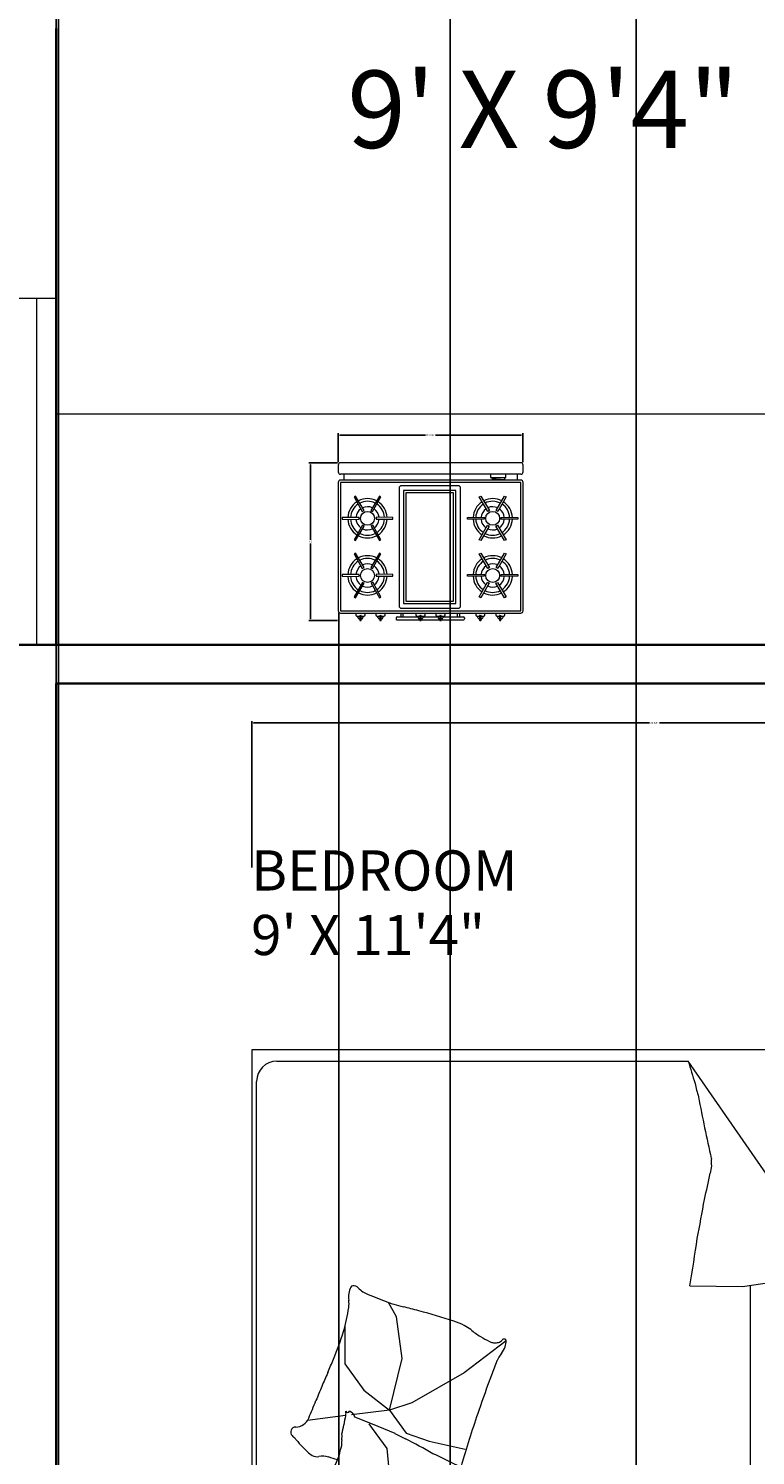
# Model space of a CAD drawing. Units: feet. Extents: x 1993 to 2298, y 2938 to 3641.
# Tile 6 of 11: x 2147 to 2222, y 3144 to 3293. Entities that reach past the tile are written whole.
import ezdxf

# ---------------------------------------------------------------- set-up
doc = ezdxf.new("R2010")
doc.units = ezdxf.units.FT
for name, color, linetype, lineweight in [('A-ANNO-DIMS', 2, 'Continuous', 18), ('A-AREA-IDEN', 7, 'Continuous', 18), ('A-EQPM', 8, 'Continuous', 18), ('A-FLOR-CASE', 8, 'Continuous', 18), ('A-GLAZ', 4, 'Continuous', 13), ('furniture', 8, 'Continuous', 18), ('WAL', 7, 'Continuous', 35)]:
    doc.layers.add(name, color=color, linetype=linetype, lineweight=lineweight)
doc.styles.add('DIM_FONT', font='SIMPLEX.shx', dxfattribs={"width": 0.8})
doc.styles.get("Standard").update_dxf_attribs({"font": 'arial.ttf'})
doc.dimstyles.get("Standard").update_dxf_attribs({"dimtxt": 0.18, "dimasz": 0.18, "dimexe": 0.18, "dimexo": 0.0625, "dimgap": 0.09, "dimtad": 0, "dimtih": 1, "dimtoh": 1, "dimdec": 4, "dimzin": 0, "dimdsep": 46, "dimtxsty": 'Standard', "dimcen": 0.09, "dimadec": 0, "dimazin": 0, "dimtfac": 1, "dimtdec": 4, "dimtofl": 0, "dimtmove": 0, "dimatfit": 3, "dimfxl": 1, "dimtolj": 1, "dimtzin": 0, "dimarcsym": 0})

# ---------------------------------------------------------------- blocks, each defined once
blk = doc.blocks.new('A$C79766A75')
for p, q in [((0.45, 1.9999), (0, 1.9999)), ((0, 1.9999), (0, 1.5499)), ((0.45, 1.5499), (0.45, 1.9999)), ((1.9506, 2), (0.4506, 2)), ((0.4506, 2), (0.4506, 0)), ((1.9506, 0), (1.9506, 2)), ((2.402, 1.9999), (1.952, 1.9999)), ((1.952, 1.9999), (1.952, 1.5499)), ((2.402, 1.5499), (2.402, 1.9999)), ((0.42, 1.9699), (0.03, 1.9699)), ((0.03, 1.9699), (0.03, 1.5799)), ((0.42, 1.5799), (0.42, 1.9699)), ((2.372, 1.9699), (1.982, 1.9699)), ((1.982, 1.9699), (1.982, 1.5799)), ((2.372, 1.5799), (2.372, 1.9699)), ((0.2304, 1.9125), (0.2304, 1.6061)), ((1.9506, 1.9476), (0.4506, 1.9476)), ((2.1824, 1.9125), (2.1824, 1.6061)), ((0.0743, 1.7595), (0.3834, 1.7595)), ((2.0263, 1.7595), (2.3354, 1.7595)), ((1.1461, 1.5617), (1.1254, 1.6443)), ((1.8553, 1.5617), (1.8346, 1.6443)), ((0.4234, 1.6034), (0.4228, 1.6034)), ((0.03, 1.5799), (0.42, 1.5799)), ((1.1536, 1.5317), (1.1461, 1.5617)), ((1.8628, 1.5317), (1.8553, 1.5617)), ((1.982, 1.5799), (2.372, 1.5799)), ((0, 1.5499), (0.45, 1.5499)), ((1.952, 1.5499), (2.402, 1.5499)), ((1.0972, 1.5115), (0.4791, 1.0841)), ((1.0972, 1.5115), (1.9048, 1.5115)), ((1.9248, 1.4915), (1.9248, 0.0322)), ((1.0383, 1.2184), (1.0246, 1.3138)), ((1.9048, 1.2389), (1.0354, 1.2389)), ((1.0365, 1.0883), (1.0383, 1.2184)), ((0.4791, 0.0622), (0.4791, 1.0841)), ((1.1731, 0.6316), (1.2523, 0.5276)), ((1.5696, 0.6317), (1.5559, 0.5286)), ((1.2523, 0.5276), (1.3274, 0.3973)), ((1.4223, 0.4407), (1.442, 0.5296)), ((1.5559, 0.5286), (1.5817, 0.4065)), ((1.6952, 0.4478), (1.7898, 0.4856)), ((1.7898, 0.4856), (1.8139, 0.4822)), ((1.4025, 0.3834), (1.4223, 0.4407)), ((1.6264, 0.355), (1.6952, 0.4478)), ((1.3274, 0.3973), (1.3452, 0.342)), ((1.5817, 0.4065), (1.6264, 0.355)), ((1.1139, 0.3597), (1.0779, 0.3397)), ((1.2167, 0.3736), (1.1139, 0.3597)), ((1.3452, 0.342), (1.2167, 0.3736)), ((1.3452, 0.342), (1.4025, 0.3834)), ((1.4034, 0.3558), (1.3803, 0.2995)), ((1.6264, 0.355), (1.4406, 0.3361)), ((1.5954, 0.2725), (1.6264, 0.355)), ((1.6264, 0.355), (1.6935, 0.3825)), ((1.6935, 0.3825), (1.7623, 0.379)), ((1.7623, 0.379), (1.8603, 0.3619)), ((1.8603, 0.3619), (1.8636, 0.3554)), ((1.2957, 0.2787), (1.3452, 0.342)), ((1.3452, 0.342), (1.3569, 0.2478)), ((1.4406, 0.3361), (1.3907, 0.3)), ((1.3803, 0.2995), (1.3626, 0.256)), ((1.3907, 0.3), (1.3787, 0.2914)), ((1.2305, 0.2313), (1.2957, 0.2787)), ((1.6161, 0.19), (1.5954, 0.2725)), ((1.1376, 0.2313), (1.2305, 0.2313)), ((1.3588, 0.2331), (1.3706, 0.1385)), ((1.6697, 0.1274), (1.6161, 0.19)), ((1.9048, 0.0122), (0.5291, 0.0122)), ((0.4506, 0), (1.9506, 0))]:
    blk.add_line(p, q)
for centre in [(0.2304, 1.7595), (2.1824, 1.7595)]:
    blk.add_circle(centre, 0.126)
for centre, radius, start, end in [((0.5232, 1.9139), 0.00342, 291.7883, 340.436), ((0.5246, 1.9378), 0.0251, 274.3025, 291.7883), ((0.5486, 1.9393), 0.0289, 239.3487, 274.3025), ((1.1179, 2.0719), 0.1611, 270, 278.4372), ((1.1592, 2.0011), 0.0904, 258.7276, 270), ((1.2325, 1.9139), 0.00342, 291.7883, 340.436), ((1.2338, 1.9378), 0.0251, 274.3025, 291.7883), ((1.2578, 1.9393), 0.0289, 239.3487, 274.3025), ((1.8271, 2.0719), 0.1611, 270, 278.4372), ((1.8684, 2.0011), 0.0904, 258.7276, 270), ((0.525, 1.9085), 0.00232, 340.436, 101.8931), ((0.5311, 1.9093), 0.00428, 201.9904, 281.8931), ((0.4996, 1.8889), 0.0328, 338.579, 8.1335), ((0.2896, 1.8253), 0.246, 8.1335, 12.1095), ((0.5465, 1.8994), 0.0156, 158.579, 201.9904), ((0.5458, 1.8568), 0.0539, 59.3487, 84.7408), ((0.546, 1.0829), 0.8208, 84.7408, 88.0921), ((0.6118, 2.0005), 0.0992, 254.0648, 274.2159), ((0.6775, 1.9817), 0.0992, 233.9136, 254.0648), ((0.6362, 0.406), 1.4943, 88.0921, 90.5757), ((0.7304, 1.9449), 0.0992, 216.1766, 233.9136), ((0.7737, 2.1075), 0.234, 242.7604, 249.1397), ((0.7591, 1.0293), 0.8732, 90.5757, 94.8018), ((0.738, 1.949), 0.0768, 231.6114, 242.7604), ((0.974, 2.1633), 0.3916, 226.1885, 231.6114), ((0.7631, 2.1919), 0.2897, 267.4614, 274.8018), ((0.8143, 2.0532), 0.1524, 259.8101, 267.4614), ((0.7515, 1.3747), 0.5293, 79.8101, 83.9133), ((0.8451, 0.8466), 1.049, 83.9133, 90), ((1.046, 1.2129), 0.6827, 90, 97.5469), ((1.1117, 1.6625), 0.2422, 97.5469, 105.744), ((1.0352, 2.2041), 0.3048, 278.4372, 285.744), ((1.171, 1.8579), 0.0342, 94.4002, 153.4195), ((1.1709, 1.9049), 0.0131, 153.4195, 258.7276), ((1.2342, 1.9085), 0.00232, 340.436, 101.8931), ((1.2404, 1.9093), 0.00428, 201.9904, 281.8931), ((1.2088, 1.8889), 0.0328, 338.579, 8.1335), ((0.9988, 1.8253), 0.246, 8.1335, 12.1095), ((1.2558, 1.8994), 0.0156, 158.579, 201.9904), ((1.2551, 1.8568), 0.0539, 59.3487, 84.7408), ((1.2552, 1.0829), 0.8208, 84.7408, 88.0921), ((1.3211, 2.0005), 0.0992, 254.0648, 274.2159), ((1.3868, 1.9817), 0.0992, 233.9136, 254.0648), ((1.3455, 0.406), 1.4943, 88.0921, 90.5757), ((1.4396, 1.9449), 0.0992, 216.1766, 233.9136), ((1.4829, 2.1075), 0.234, 242.7604, 249.1397), ((1.4683, 1.0293), 0.8732, 90.5757, 94.8018), ((1.4473, 1.949), 0.0768, 231.6114, 242.7604), ((1.6833, 2.1633), 0.3916, 226.1885, 231.6114), ((1.4724, 2.1919), 0.2897, 267.4614, 274.8018), ((1.5236, 2.0532), 0.1524, 259.8101, 267.4614), ((1.4607, 1.3747), 0.5293, 79.8101, 83.9133), ((1.5543, 0.8466), 1.049, 83.9133, 90), ((1.7552, 1.2129), 0.6827, 90, 97.5469), ((1.821, 1.6625), 0.2422, 97.5469, 105.744), ((1.7444, 2.2041), 0.3048, 278.4372, 285.744), ((1.8802, 1.8579), 0.0342, 94.4002, 153.4195), ((1.8802, 1.9049), 0.0131, 153.4195, 258.7276), ((0.7297, 1.8867), 0.1983, 187.6809, 192.1095), ((1.4472, 1.8987), 0.9131, 183.3687, 187.6809), ((0.7661, 1.8961), 0.0992, 198.4397, 216.1766), ((0.9057, 1.9982), 0.2252, 219.0349, 226.1885), ((1.6324, 1.8735), 0.4918, 180, 186.2324), ((1.4389, 1.8867), 0.1983, 187.6809, 192.1095), ((2.1565, 1.8987), 0.9131, 183.3687, 187.6809), ((1.4753, 1.8961), 0.0992, 198.4397, 216.1766), ((1.615, 1.9982), 0.2252, 219.0349, 226.1885), ((1.6908, 1.9123), 0.1399, 314.9024, 332.6012), ((1.7511, 1.9723), 0.1399, 297.2036, 314.9024), ((1.7896, 1.8667), 0.0526, 318.5571, 334.6449), ((1.784, 1.9167), 0.0899, 306.2641, 318.5571), ((2.3416, 1.8735), 0.4918, 180, 186.2324), ((0.7932, 1.8591), 0.0493, 208.3168, 219.0349), ((0.9392, 1.9062), 0.2002, 203.0028, 208.3168), ((1.3446, 1.7858), 0.204, 170.3156, 180), ((1.5025, 1.8591), 0.0493, 208.3168, 219.0349), ((1.6484, 1.9062), 0.2002, 203.0028, 208.3168), ((1.6554, 1.8529), 0.1399, 332.6012, 343.485), ((1.7653, 1.8132), 0.0562, 341.2201, 0), ((1.6307, 1.8895), 0.2056, 338.1851, 341.2201), ((1.6887, 1.8881), 0.1511, 334.6449, 338.1851), ((2.0538, 1.7858), 0.204, 170.3156, 180), ((1.2208, 1.7573), 0.6787, 178.3669, 183.3687), ((2.0027, 1.5994), 0.882, 167.8016, 170.3156), ((1.9301, 1.7573), 0.6787, 178.3669, 183.3687), ((1.6404, 1.8023), 0.1399, 343.485, 354.3689), ((1.73, 1.7719), 0.0915, 0, 14.6851), ((2.7119, 1.5994), 0.882, 167.8016, 170.3156), ((0.8192, 1.792), 0.3171, 347.8016, 351.9949), ((1.5284, 1.792), 0.3171, 347.8016, 351.9949), ((1.9066, 1.6447), 1.3652, 176.945, 178.3669), ((0.4711, 1.7556), 0.6588, 351.9949, 357.3351), ((2.6158, 1.6447), 1.3652, 176.945, 178.3669), ((1.1803, 1.7556), 0.6588, 351.9949, 357.3351), ((14.1519, 0.85), 13.6356, 176.49514, 176.94504), ((14.8612, 0.85), 13.6356, 176.49514, 176.94504), ((1.0578, 1.6474), 0.0677, 357.3351, 14.0452), ((1.767, 1.6474), 0.0677, 357.3351, 14.0452), ((0.7658, 2.8912), 1.4323, 294.3265, 296.4985), ((1.226, 2.0834), 0.5066, 290.6743, 294.3265), ((1.4305, 1.6796), 0.058, 274.0828, 290.6743), ((1.4679, 1.8969), 0.2721, 266.4448, 274.0828), ((0.8521, 1.5209), 0.3212, 170.0016, 176.4951), ((0.6583, 0.9067), 0.7387, 64.6889, 66.5156), ((0.7015, 0.888), 0.7387, 66.5156, 68.3423), ((0.7501, 0.8688), 0.7387, 68.3423, 70.572), ((1.5613, 1.5209), 0.3212, 170.0016, 176.4951), ((0.9025, 2.1618), 0.7286, 302.135, 305.8263), ((1.1895, 1.8508), 0.3126, 296.4985, 302.135), ((1.3675, 0.9067), 0.7387, 64.6889, 66.5156), ((1.4107, 0.888), 0.7387, 66.5156, 68.3423), ((1.4594, 0.8688), 0.7387, 68.3423, 70.572), ((0.513, 1.535), 0.0193, 350.0016, 16.6978), ((0.5322, 1.5304), 0.00132, 16.6978, 97.1204), ((0.5579, 1.4467), 0.0875, 97.1204, 106.2212), ((0.5822, 1.4654), 0.0767, 106.2212, 117.2841), ((0.5507, 1.5832), 0.0453, 282.869, 297.2841), ((0.5623, 1.6885), 0.1459, 273.574, 282.869), ((0.589, 2.7103), 1.164, 270.2865, 273.574), ((0.7584, 7.2662), 5.7185, 269.0296, 270.2865), ((0.9401, 4.9065), 3.3622, 267.3904, 269.0296), ((0.9811, 2.7573), 1.2165, 265.3824, 267.3904), ((0.8583, 0.139), 1.4048, 85.3824, 87.2509), ((1.0175, 1.3138), 0.2301, 87.2509, 101.5586), ((0.8043, 0.8497), 0.7387, 70.572, 72.8018), ((1.0449, 1.6886), 0.1459, 263.5659, 281.5586), ((1.1099, 1.6599), 0.1197, 252.6136, 263.5659), ((1.0587, 1.3144), 0.2297, 72.6136, 80.5159), ((1.108, 1.2635), 0.2708, 80.5159, 85.9171), ((1.1535, 1.5308), 0.000917, 85.9171, 194.0449), ((1.2222, 1.535), 0.0193, 350.0016, 16.6978), ((1.2414, 1.5304), 0.00132, 16.6978, 97.1204), ((1.2671, 1.4467), 0.0875, 97.1204, 106.2212), ((1.2914, 1.4654), 0.0767, 106.2212, 117.2841), ((1.2599, 1.5832), 0.0453, 282.869, 297.2841), ((1.2716, 1.6885), 0.1459, 273.574, 282.869), ((1.2982, 2.7103), 1.164, 270.2865, 273.574), ((1.4677, 7.2662), 5.7185, 269.0296, 270.2865), ((1.6493, 4.9065), 3.3622, 267.3904, 269.0296), ((1.6903, 2.7573), 1.2165, 265.3824, 267.3904), ((1.5676, 0.139), 1.4048, 85.3824, 87.2509), ((1.7268, 1.3138), 0.2301, 87.2509, 101.5586), ((1.5136, 0.8497), 0.7387, 70.572, 72.8018), ((1.7541, 1.6886), 0.1459, 263.5659, 281.5586), ((1.8192, 1.6599), 0.1197, 252.6136, 263.5659), ((1.7679, 1.3144), 0.2297, 72.6136, 80.5159), ((1.8172, 1.2635), 0.2708, 80.5159, 85.9171), ((1.8627, 1.5308), 0.000917, 85.9171, 194.0449), ((0.745, 1.6407), 0.3751, 320.3555, 339.8512), ((1.9048, 1.4915), 0.02, 0, 90), ((0.8556, 1.3759), 0.1801, 339.8512, 8.1356), ((1.9048, 1.2589), 0.02, 270, 0), ((-0.1888, 5.1029), 4.0646, 280.7276, 282.9255), ((0.7282, 1.1989), 0.0581, 262.2696, 280.7276), ((0.7833, 1.3309), 0.1942, 256.8096, 262.2696), ((0.2481, -1.3253), 2.5158, 76.8096, 78.3259), ((-0.0248, 2.8487), 1.8351, 285.9352, 287.7364), ((0.3872, 1.7415), 0.6574, 282.9255, 285.9352), ((0.3953, -1.4284), 2.588, 78.3259, 80.505), ((0.413, -2.64), 3.7801, 80.505, 82.308), ((1.1752, 0.6267), 0.0063, 166.7192, 233.4208), ((1.1734, 0.6272), 0.00443, 93.9484, 166.7192), ((1.163, 0.6103), 0.0142, 10.4074, 53.4208), ((1.1755, 0.5964), 0.0352, 69.6548, 93.9484), ((1.1011, 0.5989), 0.0771, 2.7286, 10.4074), ((1.1628, 0.6019), 0.0153, 345.4291, 2.7286), ((1.1669, 0.5731), 0.0601, 51.4146, 69.6548), ((1.2538, 0.682), 0.0792, 231.4146, 247.2931), ((1.5463, 1.3811), 0.8371, 247.2931, 249.8713), ((1.383, 0.7705), 0.2176, 307.2151, 313.5224), ((1.1426, 1.1456), 0.6605, 306.2163, 307.2151), ((1.7751, 0.3162), 0.3825, 126.2163, 127.5287), ((1.5806, 0.5924), 0.0452, 127.5287, 134.1274), ((1.5093, 0.6825), 0.0697, 308.8136, 314.1274), ((1.5706, 0.6318), 0.0127, 176.7545, 308.8136), ((1.5621, 0.59), 0.0359, 356.7545, 62.7098), ((0.9961, 0.6678), 0.194, 320.2995, 329.0944), ((0.8605, 0.749), 0.352, 329.0944, 333.1821), ((1.1396, 0.6079), 0.0393, 333.1821, 345.4291), ((3.0113, 5.3783), 5.0942, 249.8713, 250.9164), ((1.5435, 0.5526), 0.0458, 157.5838, 188.0492), ((1.4828, 0.5833), 0.0226, 324.1064, 8.0492), ((1.4519, 0.6426), 0.0774, 313.5224, 324.1064), ((0.2201, -2.1858), 3.0972, 62.7098, 63.5853), ((2.5711, 2.3551), 2.0162, 242.5001, 243.5853), ((1.2077, 0.4922), 0.081, 140.2995, 153.9265), ((2.374, 3.5362), 3.145, 250.9164, 253.3915), ((2.4089, 0.1204), 1.0054, 154.9471, 157.5838), ((4.5245, 5.9445), 6.1019, 242.15178, 242.50014), ((-0.9881, -4.647), 5.8383, 62.15178, 62.50792), ((3.0311, -0.112), 2.003, 162.1604, 164.7375), ((1.3115, 0.4414), 0.1965, 153.9265, 162.1604), ((2.9813, -0.2643), 1.6868, 152.9116, 154.9471), ((1.5084, 0.6341), 0.1166, 253.3915, 259.2634), ((1.5182, -0.068), 0.6236, 62.5079, 69.2514), ((1.7121, 0.0657), 0.43, 69.2514, 77.3748), ((1.8682, 0.4049), 0.063, 77.3748, 93.3881), ((1.8955, 0.5247), 0.0599, 256.9598, 273.3881), ((1.9257, 0.5082), 0.0509, 238.3083, 256.9598), ((2.8096, -0.3311), 1.5652, 150.064, 152.9116), ((1.8435, 0.4743), 0.0755, 310.5086, 333.6668), ((1.9279, 0.441), 0.0168, 130.5086, 180.9614), ((1.9201, 0.4587), 0.0058, 180.9614, 238.3083), ((2.6887, -0.0186), 1.6481, 164.7375, 166.159), ((-0.5166, 1.5491), 2.6619, 333.6668, 334.8268), ((0.5589, 0.5062), 0.5454, 343.6878, 346.159), ((1.2176, 0.4627), 0.2143, 330.064, 337.7645), ((1.3456, 0.5261), 0.5454, 339.2919, 341.7631), ((1.701, 0.4319), 0.1798, 334.8268, 339.2919), ((-1.4109, 1.284), 2.6619, 338.0627, 339.2227), ((0.9098, 0.4035), 0.1798, 339.2227, 343.6878), ((3.4079, -0.2212), 1.6481, 160.3416, 161.7631), ((0.9882, 0.3177), 0.0755, 314.9045, 338.0627), ((3.6966, -0.4634), 2.003, 157.7645, 160.3416), ((1.0533, 0.2524), 0.0168, 134.9045, 185.3572), ((1.0424, 0.2513), 0.0058, 185.3572, 242.7041), ((1.3694, 0.234), 0.0231, 107.1867, 157.7645), ((1.0631, 0.2914), 0.0509, 242.7041, 261.3557), ((1.0645, 0.3003), 0.0599, 261.3557, 277.784), ((1.0811, 0.1786), 0.063, 81.7707, 97.784), ((1.0286, -0.1846), 0.43, 73.6473, 81.7707), ((0.974, -0.3705), 0.6236, 66.9038, 73.6473), ((1.3465, 0.2383), 0.00467, 287.1867, 70.6201), ((1.3486, 0.2247), 0.0092, 70.6201, 94.2593), ((1.3563, 0.267), 0.034, 262.0178, 274.2593), ((1.4091, 0.4221), 0.1955, 255.1193, 262.0178), ((1.358, 0.0507), 0.1794, 75.1193, 82.3216), ((1.4096, 0.153), 0.0712, 82.3216, 94.5118), ((1.4285, 0.2893), 0.0663, 261.8784, 274.5118), ((1.4755, 0.332), 0.1166, 248.9957, 261.8784), ((2.7121, 3.1012), 3.145, 246.5205, 248.9957), ((2.4175, -0.1202), 1.0054, 160.6552, 161.9797), ((-1.0716, -5.1672), 5.8383, 66.54766, 66.9038), ((3.6805, 5.7866), 6.1019, 246.54766, 246.89602), ((1.505, 0.1766), 0.0458, 161.9797, 192.4451), ((1.856, 0.1288), 0.081, 135.9036, 149.5306), ((1.9797, 0.1108), 0.1965, 149.5306, 157.7645), ((2.0773, 2.0287), 2.0162, 246.896, 247.9812), ((0.1602, -2.7118), 3.0972, 67.1056, 67.9812), ((1.3914, 0.1905), 0.0774, 317.9183, 328.5023), ((1.4382, 0.1619), 0.0226, 328.5023, 12.4451), ((3.6993, 4.7998), 5.0942, 245.4754, 246.5205), ((1.4661, 0.3294), 0.352, 324.6985, 328.7862), ((1.6279, 0.2819), 0.194, 315.9036, 324.6985), ((1.3512, 0.1084), 0.0359, 1.1504, 67.1056), ((1.3997, 0.1094), 0.0127, 181.1504, 313.2095), ((1.4468, 0.0748), 0.0452, 131.9246, 138.5233), ((1.6722, -0.1762), 0.3825, 130.6122, 131.9246), ((0.9933, 0.6156), 0.6605, 310.6122, 311.611), ((1.2874, 0.2845), 0.2176, 311.611, 317.9183), ((2.051, 0.8725), 0.8371, 242.8972, 245.4754), ((1.7576, 0.1689), 0.0792, 227.0187, 242.8972), ((1.7345, 0.1188), 0.0153, 341.0332, 358.3327), ((1.6723, 0.1058), 0.0771, 358.3327, 6.0115), ((1.7162, 0.1388), 0.0393, 328.7862, 341.0332), ((1.3607, 0.1509), 0.0697, 313.2095, 318.5233), ((1.6963, 0.0438), 0.0601, 47.0187, 65.2589), ((1.737, 0.0526), 0.0352, 65.2589, 89.5525), ((1.7401, 0.0928), 0.0142, 6.0115, 49.0249), ((1.756, 0.0832), 0.00443, 89.5525, 162.3233), ((1.7602, 0.0924), 0.0063, 162.3233, 229.0249), ((0.5291, 0.0622), 0.05, 180, 270), ((1.9048, 0.0322), 0.02, 270, 0)]:
    blk.add_arc(centre, radius, start, end)
at = {"style": 'DIM_FONT', "text_generation_flag": 4, "width": 0.8, "flags": 9}
for tag in ['XSIZE', 'YSIZE']:
    blk.add_attdef(tag, (1.9506, 2), '', height=0.0005, rotation=180, dxfattribs=at)
blk = doc.blocks.new('A$C389D7A6F')
for p, q in [((790, 682.5), (10, 682.5)), ((0, 672.5), (0, 642.5)), ((790, 632.5), (10, 632.5)), ((25, 632.5), (25, 607.5)), ((659, 632.5), (659, 618)), ((659, 618), (726.2, 618)), ((664.5, 618), (664.5, 614.8)), ((721.4, 609.3), (721, 618)), ((726.2, 618), (726.2, 632.5)), ((775, 632.5), (775, 607.5)), ((800, 642.5), (800, 672.5)), ((0, 597.5), (0, 42.5)), ((790, 607.5), (10, 607.5)), ((790, 597.5), (10, 597.5)), ((10, 597.5), (10, 42.5)), ((263.3, 572.9), (263.3, 63.4)), ((519.8, 582.9), (273.3, 582.9)), ((509.8, 562.9), (283.3, 562.9)), ((283.3, 562.9), (283.3, 73.4)), ((509.8, 73.4), (509.8, 562.9)), ((529.8, 63.4), (529.8, 572.9)), ((664.5, 614.8), (721.4, 609.3)), ((790, 42.5), (790, 597.5)), ((800, 42.5), (800, 597.5)), ((75.6, 538.6), (69.3, 534.9)), ((69.3, 534.9), (104.4, 471.6)), ((111.8, 475.9), (75.6, 538.6)), ((178.4, 538.6), (141.2, 476.5)), ((148.6, 472.2), (184.8, 534.9)), ((184.8, 534.9), (178.4, 538.6)), ((499.8, 552.9), (293.3, 552.9)), ((293.3, 552.9), (293.3, 83.4)), ((499.8, 83.4), (499.8, 552.9)), ((610.9, 534.9), (617.2, 538.6)), ((647.1, 472.2), (610.9, 534.9)), ((617.2, 538.6), (654.5, 476.5)), ((683.9, 475.9), (720, 538.6)), ((726.4, 534.9), (691.3, 471.6)), ((720, 538.6), (726.4, 534.9)), ((90.2, 445.9), (17.9, 445.9)), ((17.9, 445.9), (17.9, 438.5)), ((17.9, 438.5), (90.2, 437.3)), ((90.2, 437.3), (90.2, 445.9)), ((104.4, 471.6), (111.8, 475.9)), ((141.2, 476.5), (148.6, 472.2)), ((236.2, 445.9), (163.8, 447.1)), ((163.8, 447.1), (163.8, 438.5)), ((163.8, 438.5), (236.2, 438.5)), ((236.2, 438.6), (236.2, 445.9)), ((559.5, 445.9), (631.8, 447.1)), ((559.5, 438.6), (559.5, 445.9)), ((631.8, 438.5), (559.5, 438.5)), ((631.8, 447.1), (631.8, 438.5)), ((654.5, 476.5), (647.1, 472.2)), ((691.3, 471.6), (683.9, 475.9)), ((705.4, 445.9), (777.8, 445.9)), ((705.4, 437.3), (705.4, 445.9)), ((777.8, 438.5), (705.4, 437.3)), ((777.8, 445.9), (777.8, 438.5)), ((105.4, 412.2), (69.3, 349.5)), ((75.6, 345.8), (112.9, 407.9)), ((112.9, 407.9), (105.4, 412.2)), ((149.7, 412.8), (142.3, 408.5)), ((142.3, 408.5), (178.4, 345.8)), ((184.8, 349.5), (149.7, 412.8)), ((610.9, 349.5), (646, 412.8)), ((653.4, 408.5), (617.2, 345.8)), ((646, 412.8), (653.4, 408.5)), ((682.8, 407.9), (690.2, 412.2)), ((720, 345.8), (682.8, 407.9)), ((690.2, 412.2), (726.4, 349.5)), ((69.3, 349.5), (75.6, 345.8)), ((178.4, 345.8), (184.8, 349.5)), ((617.2, 345.8), (610.9, 349.5)), ((726.4, 349.5), (720, 345.8)), ((75.6, 291.6), (69.3, 287.9)), ((69.3, 287.9), (104.4, 224.6)), ((111.8, 228.9), (75.6, 291.6)), ((178.4, 291.6), (141.2, 229.5)), ((148.6, 225.2), (184.8, 287.9)), ((184.8, 287.9), (178.4, 291.6)), ((610.9, 287.9), (617.2, 291.6)), ((647.1, 225.2), (610.9, 287.9)), ((617.2, 291.6), (654.5, 229.5)), ((683.9, 228.9), (720, 291.6)), ((726.4, 287.9), (691.3, 224.6)), ((720, 291.6), (726.4, 287.9)), ((17.9, 198.9), (17.9, 191.5)), ((90.2, 198.9), (17.9, 198.9)), ((17.9, 191.5), (90.2, 190.3)), ((90.2, 190.3), (90.2, 198.9)), ((104.4, 224.6), (111.8, 228.9)), ((141.2, 229.5), (148.6, 225.2)), ((163.8, 200.1), (163.8, 191.5)), ((236.2, 198.9), (163.8, 200.1)), ((163.8, 191.5), (236.2, 191.5)), ((236.2, 191.6), (236.2, 199)), ((559.5, 198.9), (631.8, 200.1)), ((559.5, 191.4), (559.5, 198.8)), ((631.8, 191.5), (559.5, 191.5)), ((631.8, 200.1), (631.8, 191.5)), ((654.5, 229.5), (647.1, 225.2)), ((691.3, 224.6), (683.9, 228.9)), ((705.4, 190.3), (705.4, 198.9)), ((705.4, 198.9), (777.8, 198.9)), ((777.8, 191.5), (705.4, 190.3)), ((777.8, 198.9), (777.8, 191.5)), ((105.4, 165.2), (69.3, 102.5)), ((75.6, 98.8), (112.9, 160.9)), ((112.9, 160.9), (105.4, 165.2)), ((149.7, 165.8), (142.3, 161.5)), ((142.3, 161.5), (178.4, 98.8)), ((184.8, 102.5), (149.7, 165.8)), ((610.9, 102.5), (646, 165.8)), ((653.4, 161.5), (617.2, 98.8)), ((646, 165.8), (653.4, 161.5)), ((682.8, 160.9), (690.2, 165.2)), ((720, 98.8), (682.8, 160.9)), ((690.2, 165.2), (726.4, 102.5)), ((69.3, 102.5), (75.6, 98.8)), ((178.4, 98.8), (184.8, 102.5)), ((283.3, 73.4), (509.8, 73.4)), ((293.3, 83.4), (499.8, 83.4)), ((617.2, 98.8), (610.9, 102.5)), ((726.4, 102.5), (720, 98.8)), ((10, 42.5), (790, 42.5)), ((10, 32.5), (790, 32.5)), ((76.4, 32.5), (76.4, 24.4)), ((81.4, 19.4), (93.4, 19.4)), ((93.4, 21.3), (93.4, 1)), ((94.4, 22.3), (98.3, 22.3)), ((94.4, 0), (98.3, 0)), ((99.3, 1), (99.3, 21.3)), ((99.3, 19.4), (111.4, 19.4)), ((116.4, 24.4), (116.4, 32.5)), ((162.8, 32.5), (162.8, 24.4)), ((167.8, 19.4), (179.8, 19.4)), ((179.8, 21.3), (179.8, 1)), ((180.8, 22.3), (184.7, 22.3)), ((180.8, 0), (184.7, 0)), ((185.7, 1), (185.7, 21.3)), ((185.7, 19.4), (197.8, 19.4)), ((202.8, 24.4), (202.8, 32.5)), ((250.6, 11), (250.6, 7.3)), ((255.6, 16), (343.8, 16)), ((353.5, 2.3), (255.6, 2.3)), ((270.6, 32.5), (270.6, 16)), ((273.3, 53.4), (519.8, 53.4)), ((280.6, 16), (280.6, 32.5)), ((336.4, 32.5), (336.4, 24.4)), ((341.4, 19.4), (353.5, 19.4)), ((353.5, 21.3), (353.5, 1)), ((354.5, 22.3), (358.4, 22.3)), ((354.5, 0), (358.4, 0)), ((359.4, 1), (359.4, 21.3)), ((359.4, 19.4), (371.4, 19.4)), ((440, 2.3), (359.4, 2.3)), ((369.1, 16), (430.4, 16)), ((376.4, 24.4), (376.4, 32.5)), ((423, 32.5), (423, 24.4)), ((428, 19.4), (440, 19.4)), ((440, 21.3), (440, 1)), ((441, 22.3), (444.9, 22.3)), ((441, 0), (444.9, 0)), ((445.9, 1), (445.9, 21.3)), ((445.9, 19.4), (458, 19.4)), ((541.8, 2.3), (445.9, 2.3)), ((455.6, 16), (541.8, 16)), ((463, 24.4), (463, 32.5)), ((515.8, 16), (515.8, 32.5)), ((525.8, 32.5), (525.8, 16)), ((546.8, 11), (546.8, 7.3)), ((595.2, 32.5), (595.2, 24.4)), ((600.2, 19.4), (612.3, 19.4)), ((612.3, 21.3), (612.3, 1)), ((613.3, 22.3), (617.2, 22.3)), ((613.3, 0), (617.2, 0)), ((618.2, 1), (618.2, 21.3)), ((618.2, 19.4), (630.2, 19.4)), ((635.2, 24.4), (635.2, 32.5)), ((681.7, 32.5), (681.7, 24.4)), ((686.7, 19.4), (698.7, 19.4)), ((698.7, 21.3), (698.7, 1)), ((699.7, 22.3), (703.6, 22.3)), ((699.7, 0), (703.6, 0)), ((704.6, 1), (704.6, 21.3)), ((704.6, 19.4), (716.7, 19.4)), ((721.7, 24.4), (721.7, 32.5))]:
    blk.add_line(p, q)
for centre in [(127, 442), (668.7, 442), (127, 195), (668.7, 195)]:
    blk.add_circle(centre, 30.2)
for centre, radius, start, end in [((10, 672.5), 10, 90, 180), ((790, 672.5), 10, 0, 90), ((10, 642.5), 10, 180, 270), ((790, 642.5), 10, 270, 0), ((10, 597.5), 10, 90, 180), ((273.3, 572.9), 10, 90, 180), ((519.8, 572.9), 10, 0, 90), ((790, 597.5), 10, 0, 90), ((126.8, 442.3), 85, 122.64753, 177.58), ((127, 442.2), 73.6, 123.33754, 177.13402), ((126.8, 442.3), 85, 62.58907, 117.41028), ((127, 442.2), 73.6, 63.33754, 117.13402), ((127, 442.2), 73.6, 3.33754, 57.13402), ((126.8, 442.3), 85, 2.7, 57.34914), ((668.9, 442.3), 85, 122.65086, 177.3), ((668.6, 442.2), 73.6, 122.86598, 176.66246), ((668.9, 442.3), 85, 62.58972, 117.41093), ((668.6, 442.2), 73.6, 62.86598, 116.66246), ((668.6, 442.2), 73.6, 2.86598, 56.66246), ((668.9, 442.3), 85, 2.42, 57.35247), ((126.8, 442.3), 85, 182.81695, 237.68856), ((127, 442.2), 73.6, 183.33754, 237.13402), ((127, 442), 50.3, 125.13945, 175.5702), ((127, 442), 50.3, 185.097, 235.76905), ((127, 442), 50.3, 65.37866, 115.60828), ((127, 442), 50.3, 5.57548, 55.84519), ((127, 442), 50.3, 305.53298, 356.04398), ((127, 442.2), 73.6, 303.33754, 357.13402), ((126.8, 442.3), 85, 302.86942, 357.45772), ((668.9, 442.3), 85, 182.54228, 237.13058), ((668.6, 442.2), 73.6, 182.86598, 236.66246), ((668.7, 442), 50.3, 183.95602, 234.46702), ((668.7, 442), 50.3, 124.15481, 174.42452), ((668.7, 442), 50.3, 64.39172, 114.62134), ((668.7, 442), 50.3, 304.23095, 354.903), ((668.7, 442), 50.3, 4.4298, 54.86055), ((668.6, 442.2), 73.6, 302.86598, 356.66246), ((668.9, 442.3), 85, 302.31144, 357.18305), ((127, 442.2), 73.6, 243.33754, 297.13402), ((127, 442), 50.3, 245.29371, 296.00592), ((668.6, 442.2), 73.6, 242.86598, 296.66246), ((668.7, 442), 50.3, 243.99408, 294.70629), ((126.8, 442.3), 85, 242.92791, 297.62742), ((668.9, 442.3), 85, 242.37258, 297.07209), ((126.8, 195.3), 85, 122.64753, 177.58), ((127, 195.2), 73.6, 123.33754, 177.13402), ((126.8, 195.3), 85, 62.58907, 117.41028), ((127, 195.2), 73.6, 63.33754, 117.13402), ((127, 195.2), 73.6, 3.33754, 57.13402), ((126.8, 195.3), 85, 2.7, 57.34914), ((668.9, 195.3), 85, 122.65086, 177.3), ((668.6, 195.2), 73.6, 122.86598, 176.66246), ((668.9, 195.3), 85, 62.58972, 117.41093), ((668.6, 195.2), 73.6, 62.86598, 116.66246), ((668.6, 195.2), 73.6, 2.86598, 56.66246), ((668.9, 195.3), 85, 2.42, 57.35247), ((126.8, 195.3), 85, 182.81695, 237.68856), ((127, 195.2), 73.6, 183.33754, 237.13402), ((127, 195), 50.3, 125.13945, 175.5702), ((127, 195), 50.3, 185.097, 235.76905), ((127, 195), 50.3, 65.37866, 115.60828), ((127, 195), 50.3, 5.57548, 55.84519), ((127, 195), 50.3, 305.53298, 356.04398), ((127, 195.2), 73.6, 303.33754, 357.13402), ((126.8, 195.3), 85, 302.86942, 357.45772), ((668.9, 195.3), 85, 182.54228, 237.13058), ((668.6, 195.2), 73.6, 182.86598, 236.66246), ((668.7, 195), 50.3, 183.95602, 234.46702), ((668.7, 195), 50.3, 124.15481, 174.42452), ((668.7, 195), 50.3, 64.39172, 114.62134), ((668.7, 195), 50.3, 304.23095, 354.903), ((668.7, 195), 50.3, 4.4298, 54.86055), ((668.6, 195.2), 73.6, 302.86598, 356.66246), ((668.9, 195.3), 85, 302.31144, 357.18305), ((127, 195.2), 73.6, 243.33754, 297.13402), ((127, 195), 50.3, 245.29371, 296.00592), ((668.6, 195.2), 73.6, 242.86598, 296.66246), ((668.7, 195), 50.3, 243.99408, 294.70629), ((126.8, 195.3), 85, 242.92791, 297.62742), ((273.3, 63.4), 10, 180, 270), ((519.8, 63.4), 10, 270, 0), ((668.9, 195.3), 85, 242.37258, 297.07209), ((10, 42.5), 10, 180, 270), ((81.4, 24.4), 5, 180, 270), ((96.4, 18.8), 12.9, 177.39525, 256.86344), ((94.4, 21.3), 1, 90, 180), ((94.4, 1), 1, 180, 270), ((98.3, 21.3), 1, 0, 90), ((98.3, 1), 1, 270, 0), ((96.4, 18.8), 12.9, 283.13656, 2.60475), ((111.4, 24.4), 5, 270, 0), ((167.8, 24.4), 5, 180, 270), ((182.8, 18.8), 12.9, 177.39525, 256.86344), ((180.8, 21.3), 1, 90, 180), ((180.8, 1), 1, 180, 270), ((184.7, 21.3), 1, 0, 90), ((184.7, 1), 1, 270, 0), ((182.8, 18.8), 12.9, 283.13656, 2.60475), ((197.8, 24.4), 5, 270, 0), ((255.6, 11), 5, 90, 180), ((255.6, 7.3), 5, 180, 270), ((251.6, 3.3), 1, 180, 270), ((341.4, 24.4), 5, 180, 270), ((356.4, 18.8), 12.9, 177.39525, 256.86344), ((354.5, 21.3), 1, 90, 180), ((354.5, 1), 1, 180, 270), ((358.4, 21.3), 1, 0, 90), ((358.4, 1), 1, 270, 0), ((356.4, 18.8), 12.9, 283.13656, 2.60475), ((371.4, 24.4), 5, 270, 0), ((428, 24.4), 5, 180, 270), ((443, 18.8), 12.9, 177.39525, 256.86344), ((441, 21.3), 1, 90, 180), ((441, 1), 1, 180, 270), ((444.9, 21.3), 1, 0, 90), ((444.9, 1), 1, 270, 0), ((443, 18.8), 12.9, 283.13656, 2.60475), ((458, 24.4), 5, 270, 0), ((541.8, 11), 5, 0, 90), ((541.8, 7.3), 5, 270, 0), ((600.2, 24.4), 5, 180, 270), ((615.2, 18.8), 12.9, 177.39525, 256.86344), ((613.3, 21.3), 1, 90, 180), ((613.3, 1), 1, 180, 270), ((617.2, 21.3), 1, 0, 90), ((617.2, 1), 1, 270, 0), ((615.2, 18.8), 12.9, 283.13656, 2.60475), ((630.2, 24.4), 5, 270, 0), ((686.7, 24.4), 5, 180, 270), ((701.7, 18.8), 12.9, 177.39525, 256.86344), ((699.7, 21.3), 1, 90, 180), ((699.7, 1), 1, 180, 270), ((703.6, 21.3), 1, 0, 90), ((703.6, 1), 1, 270, 0), ((701.7, 18.8), 12.9, 283.13656, 2.60475), ((716.7, 24.4), 5, 270, 0), ((790, 42.5), 10, 270, 0)]:
    blk.add_arc(centre, radius, start, end)
blk = doc.blocks.new('*D31')
at = {"layer": 'A-ANNO-DIMS', "color": 0, "lineweight": -2, "transparency": 16777216}
for p, q in [((2170.07, 3205.42), (2170.07, 3220.61)), ((2170.25, 3220.43), (2211.39, 3220.43)), ((2253.58, 3220.43), (2212.44, 3220.43)), ((2253.76, 3205.42), (2253.76, 3220.61))]:
    blk.add_line(p, q, dxfattribs=at)
at = {"layer": 'A-ANNO-DIMS', "color": 0, "transparency": 16777216}
for points in [[(2170.25, 3220.46), (2170.25, 3220.4), (2170.07, 3220.43)], [(2253.58, 3220.46), (2253.58, 3220.4), (2253.76, 3220.43)]]:
    blk.add_solid(points, dxfattribs=at)
at = {"layer": 'Defpoints', "color": 0, "transparency": 16777216}
for p in [(2253.76, 3220.43), (2170.07, 3205.36), (2253.76, 3205.36)]:
    blk.add_point(p, dxfattribs=at)
at = {"layer": 'A-ANNO-DIMS', "color": 0, "transparency": 16777216, "insert": (2211.92, 3220.43), "char_height": 0.18, "attachment_point": 5}
blk.add_mtext('\\A1;84 TYP.', dxfattribs=at)
blk = doc.blocks.new('*D50')
at = {"layer": 'A-ANNO-DIMS', "color": 0, "lineweight": -2, "transparency": 16777216}
for p, q in [((2179.05, 3247.51), (2179.05, 3250.51)), ((2179.23, 3250.33), (2188.13, 3250.33)), ((2198.07, 3250.33), (2189.17, 3250.33)), ((2198.25, 3247.51), (2198.25, 3250.51))]:
    blk.add_line(p, q, dxfattribs=at)
at = {"layer": 'A-ANNO-DIMS', "color": 0, "transparency": 16777216}
for points in [[(2179.23, 3250.36), (2179.23, 3250.3), (2179.05, 3250.33)], [(2198.07, 3250.36), (2198.07, 3250.3), (2198.25, 3250.33)]]:
    blk.add_solid(points, dxfattribs=at)
at = {"layer": 'Defpoints', "color": 0, "transparency": 16777216}
for p in [(2198.25, 3250.33), (2179.05, 3247.45), (2198.25, 3247.45)]:
    blk.add_point(p, dxfattribs=at)
at = {"layer": 'A-ANNO-DIMS', "color": 0, "transparency": 16777216, "insert": (2188.65, 3250.33), "char_height": 0.18, "attachment_point": 5}
blk.add_mtext('\\A1;HOB 19', dxfattribs=at)
blk = doc.blocks.new('*D51')
at = {"layer": 'A-ANNO-DIMS', "color": 0, "lineweight": -2, "transparency": 16777216}
for p, q in [((2178.99, 3247.45), (2175.99, 3247.45)), ((2176.17, 3247.27), (2176.17, 3239.44)), ((2176.17, 3231.25), (2176.17, 3239.08)), ((2178.99, 3231.07), (2175.99, 3231.07))]:
    blk.add_line(p, q, dxfattribs=at)
at = {"layer": 'A-ANNO-DIMS', "color": 0, "transparency": 16777216}
for points in [[(2176.14, 3247.27), (2176.2, 3247.27), (2176.17, 3247.45)], [(2176.14, 3231.25), (2176.2, 3231.25), (2176.17, 3231.07)]]:
    blk.add_solid(points, dxfattribs=at)
at = {"layer": 'Defpoints', "color": 0, "transparency": 16777216}
for p in [(2176.17, 3247.45), (2179.05, 3247.45), (2179.05, 3231.07)]:
    blk.add_point(p, dxfattribs=at)
at = {"layer": 'A-ANNO-DIMS', "color": 0, "transparency": 16777216, "insert": (2176.17, 3239.26), "char_height": 0.18, "attachment_point": 5}
blk.add_mtext('\\A1;16', dxfattribs=at)
blk = doc.blocks.new('*D59')
at = {"layer": 'A-ANNO-DIMS', "color": 0, "lineweight": -2, "transparency": 16777216}
for p, q in [((2140, 3048.6), (2140, 3640.68)), ((2140.18, 3640.5), (2144.79, 3640.5)), ((2149.82, 3640.5), (2145.21, 3640.5)), ((2150, 3048.6), (2150, 3640.68))]:
    blk.add_line(p, q, dxfattribs=at)
at = {"layer": 'A-ANNO-DIMS', "color": 0, "transparency": 16777216}
for points in [[(2140.18, 3640.53), (2140.18, 3640.47), (2140, 3640.5)], [(2149.82, 3640.53), (2149.82, 3640.47), (2150, 3640.5)]]:
    blk.add_solid(points, dxfattribs=at)
at = {"layer": 'Defpoints', "color": 0, "transparency": 16777216}
for p in [(2150, 3640.5), (2140, 3048.53), (2150, 3048.53)]:
    blk.add_point(p, dxfattribs=at)
at = {"layer": 'A-ANNO-DIMS', "color": 0, "transparency": 16777216, "insert": (2145, 3640.5), "char_height": 0.18, "attachment_point": 5}
blk.add_mtext('\\A1;10', dxfattribs=at)
blk = doc.blocks.new('*D65')
at = {"layer": 'A-ANNO-DIMS', "color": 0, "lineweight": -2, "transparency": 16777216}
for p, q in [((2179.12, 3231.85), (2179.12, 2937.86)), ((2149.76, 3228.47), (2149.76, 2937.86)), ((2149.94, 2938.03), (2164.04, 2938.03)), ((2178.94, 2938.03), (2164.83, 2938.03))]:
    blk.add_line(p, q, dxfattribs=at)
at = {"layer": 'A-ANNO-DIMS', "color": 0, "transparency": 16777216}
for points in [[(2149.94, 2938.07), (2149.94, 2938.01), (2149.76, 2938.03)], [(2178.94, 2938.07), (2178.94, 2938.01), (2179.12, 2938.03)]]:
    blk.add_solid(points, dxfattribs=at)
at = {"layer": 'Defpoints', "color": 0, "transparency": 16777216}
for p in [(2179.12, 3231.92), (2149.76, 3228.53), (2179.12, 2938.03)]:
    blk.add_point(p, dxfattribs=at)
at = {"layer": 'A-ANNO-DIMS', "color": 0, "transparency": 16777216, "insert": (2164.44, 2938.03), "char_height": 0.18, "attachment_point": 5}
blk.add_mtext('\\A1;29.36', dxfattribs=at)
blk = doc.blocks.new('*D69')
at = {"layer": 'A-ANNO-DIMS', "color": 0, "lineweight": -2, "transparency": 16777216}
for p, q in [((2149.76, 3492.27), (2149.76, 2937.86)), ((2190.69, 3492.27), (2190.69, 2937.86)), ((2149.94, 2938.03), (2169.83, 2938.03)), ((2190.51, 2938.03), (2170.62, 2938.03))]:
    blk.add_line(p, q, dxfattribs=at)
at = {"layer": 'A-ANNO-DIMS', "color": 0, "transparency": 16777216}
for points in [[(2149.94, 2938.07), (2149.94, 2938.01), (2149.76, 2938.03)], [(2190.51, 2938.07), (2190.51, 2938.01), (2190.69, 2938.03)]]:
    blk.add_solid(points, dxfattribs=at)
at = {"layer": 'Defpoints', "color": 0, "transparency": 16777216}
for p in [(2149.76, 3492.33), (2190.69, 3492.33), (2190.69, 2938.03)]:
    blk.add_point(p, dxfattribs=at)
at = {"layer": 'A-ANNO-DIMS', "color": 0, "transparency": 16777216, "insert": (2170.23, 2938.03), "char_height": 0.18, "attachment_point": 5}
blk.add_mtext('\\A1;40.93', dxfattribs=at)
blk = doc.blocks.new('*D73')
at = {"layer": 'A-ANNO-DIMS', "color": 0, "lineweight": -2, "transparency": 16777216}
for p, q in [((2149.76, 3105.6), (2149.76, 3640.68)), ((2149.94, 3640.5), (2179.49, 3640.5)), ((2209.82, 3640.5), (2180.27, 3640.5)), ((2210, 3105.6), (2210, 3640.68))]:
    blk.add_line(p, q, dxfattribs=at)
at = {"layer": 'A-ANNO-DIMS', "color": 0, "transparency": 16777216}
for points in [[(2149.94, 3640.53), (2149.94, 3640.47), (2149.76, 3640.5)], [(2209.82, 3640.53), (2209.82, 3640.47), (2210, 3640.5)]]:
    blk.add_solid(points, dxfattribs=at)
at = {"layer": 'Defpoints', "color": 0, "transparency": 16777216}
for p in [(2210, 3640.5), (2149.76, 3105.53), (2210, 3105.53)]:
    blk.add_point(p, dxfattribs=at)
at = {"layer": 'A-ANNO-DIMS', "color": 0, "transparency": 16777216, "insert": (2179.88, 3640.5), "char_height": 0.18, "attachment_point": 5}
blk.add_mtext('\\A1;60.24', dxfattribs=at)

msp = doc.modelspace()

# ---------------------------------------------------------------- linework, layer by layer
at = {"layer": 'A-FLOR-CASE'}
msp.add_line((2149.7583, 3252.5338), (2257.7583, 3252.5338), dxfattribs=at)
at = {"layer": 'A-GLAZ'}
for p, q in [((2145.7583, 3264.5338), (2149.7583, 3264.5338)), ((2147.7583, 3228.5338), (2147.7583, 3264.5338))]:
    msp.add_line(p, q, dxfattribs=at)
at = {"layer": 'WAL'}
for p, q in [((2149.7583, 3228.5338), (2149.7583, 3292.5338)), ((2145.7583, 3228.5338), (2257.7583, 3228.5338)), ((2149.7583, 3088.5338), (2149.7583, 3224.5338)), ((2149.7583, 3224.5338), (2257.7583, 3224.5338))]:
    msp.add_line(p, q, dxfattribs=at)

# ---------------------------------------------------------------- block references
at = {"layer": 'A-EQPM', "xscale": 0.0240052998196229, "yscale": 0.0240052998196229, "zscale": 0.0240052998196229}
msp.add_blockref('A$C389D7A6F', (2179.0485, 3231.0665), dxfattribs=at)
at = {"layer": 'furniture', "xscale": 41.83725109546206, "yscale": 41.83725109546206, "zscale": 41.83725109546206, "rotation": 270}
msp.add_blockref('A$C79766A75', (2170.0686, 3205.3572), dxfattribs=at)

# ---------------------------------------------------------------- texts
at = {"layer": 'A-AREA-IDEN'}
for s, height, p in [('9\' X 9\'4"', 8.02685, (2180, 3280.1369)), ('BEDROOM', 4.17051, (2170, 3203.0313)), ('9\' X 11\'4"', 4.17051, (2170, 3196.3318))]:
    msp.add_text(s, height=height, dxfattribs=at).set_placement(p)

# ---------------------------------------------------------------- dimensions: what is measured, and where the dimension line sits
at = {"layer": 'A-ANNO-DIMS'}
for base, p1, p2, override, picture, middle in [((2150, 3640.4988), (2140, 3048.5338), (2150, 3048.5338), {"dimdec": 0, "dimlfac": 1, "dimrnd": 0, "dimzin": 0, "dimdsep": 46, "dimlunit": 2}, '*D59', (2145, 3640.4988)), ((2210, 3640.4988), (2149.7583, 3105.5338), (2210, 3105.5338), {"dimdec": 2, "dimlfac": 1, "dimrnd": 0, "dimzin": 0, "dimdsep": 46, "dimlunit": 2}, '*D73', (2179.8792, 3640.4988)), ((2190.6917, 2938.035), (2149.7583, 3492.3338), (2190.6917, 3492.3338), {"dimdec": 2, "dimlfac": 1, "dimrnd": 0, "dimzin": 0, "dimdsep": 46, "dimlunit": 2}, '*D69', (2170.225, 2938.035)), ((2179.1188, 2938.035), (2149.7583, 3228.5338), (2179.1188, 3231.9167), {"dimdec": 2, "dimlfac": 1, "dimrnd": 0, "dimzin": 0, "dimdsep": 46, "dimlunit": 2}, '*D65', (2164.4386, 2938.035))]:
    dim = msp.add_linear_dim(base=base, p1=p1, p2=p2, dimstyle='Standard', override=override, dxfattribs=at)
    dim.commit()
    dim.dimension.update_dxf_attribs({"geometry": picture, "text_midpoint": middle})
for base, p1, p2, text, picture, middle in [((2198.2527, 3250.3304), (2179.0485, 3247.4498), (2198.2527, 3247.4498), 'HOB <>', '*D50', (2188.6506, 3250.3304)), ((2253.764, 3220.431), (2170.0686, 3205.3572), (2253.764, 3205.3572), '<> TYP.', '*D31', (2211.9163, 3220.431))]:
    dim = msp.add_linear_dim(base=base, p1=p1, p2=p2, text=text, dimstyle='Standard', override={"dimdec": 0, "dimlfac": 1, "dimrnd": 0, "dimzin": 0, "dimdsep": 46, "dimlunit": 2}, dxfattribs=at)
    dim.commit()
    dim.dimension.update_dxf_attribs({"geometry": picture, "text_midpoint": middle})
dim = msp.add_linear_dim(base=(2176.1679, 3247.4498), p1=(2179.0485, 3231.0665), p2=(2179.0485, 3247.4498), angle=90, dimstyle='Standard', override={"dimdec": 0, "dimlfac": 1, "dimrnd": 0, "dimzin": 0, "dimdsep": 46, "dimlunit": 2}, dxfattribs=at)
dim.commit()
dim.dimension.update_dxf_attribs({"geometry": '*D51', "text_midpoint": (2176.1679, 3239.2581)})

doc.saveas('drawing.dxf')
